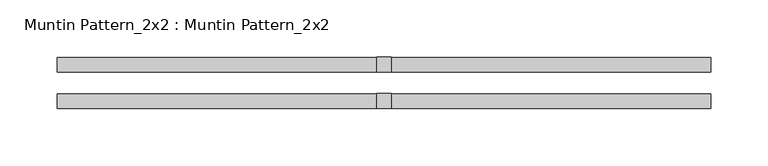
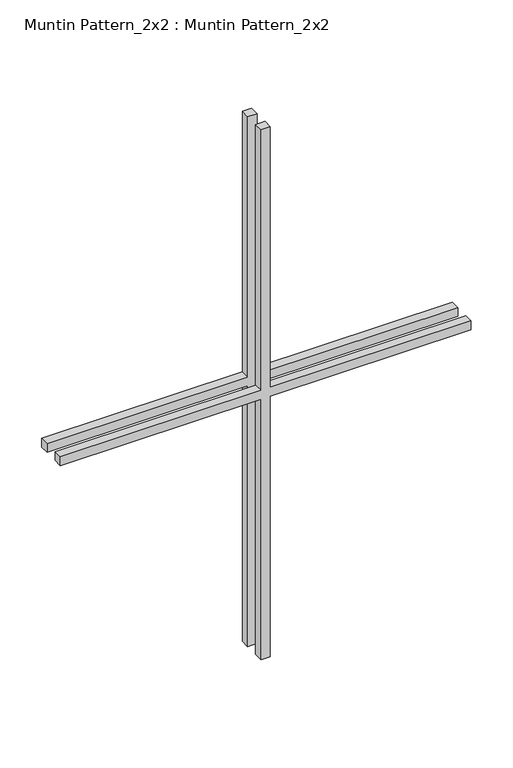
"""IFC4 building model written with IfcOpenShell, lengths in millimetres: proxy geometry, Muntin Pattern_2x2 : Muntin Pattern_2x2."""

from ifc_helpers import new_model, si_unit, frame, origin, place, context, project, spatial, polyline, outline, extrude, source, transform, mapped, element, save


def muntin_pattern_2x2_muntin_pattern_2x2_fbb866f2(model_context):
    return source(origin(), model_context, "Body", "SweptSolid", [
        extrude(outline(polyline([(393.7, -6.35), (393.7, -284.1625), (381.0, -284.1625), (381.0, -6.35), (0.0, -6.35), (0.0, 6.35), (381.0, 6.35), (381.0, 284.1625), (393.7, 284.1625), (393.7, 6.35), (774.7, 6.35), (774.7, -6.35), (393.7, -6.35)])), frame((0.0, -22.225, 0.0), z_axis=(0.0, 1.0, 0.0), x_axis=(0.0, 0.0, 1.0)), (0.0, 0.0, 1.0), 12.7),
        extrude(outline(polyline([(393.7, -6.35), (393.7, -284.1625), (381.0, -284.1625), (381.0, -6.35), (0.0, -6.35), (0.0, 6.35), (381.0, 6.35), (381.0, 284.1625), (393.7, 284.1625), (393.7, 6.35), (774.7, 6.35), (774.7, -6.35), (393.7, -6.35)])), frame((0.0, 9.525, 0.0), z_axis=(0.0, 1.0, 0.0), x_axis=(0.0, 0.0, 1.0)), (0.0, 0.0, 1.0), 12.7),
    ])


if __name__ == "__main__":
    model = new_model("IFC4")
    model_context = context("Model", 3, world=origin())
    ifc_project = project(units=[si_unit("LENGTHUNIT", "METRE", prefix="MILLI")], contexts=[model_context])
    site = spatial("IfcSite", under=ifc_project)
    building = spatial("IfcBuilding", under=site)
    placement = place(None, origin())
    muntin_pattern_2x2_muntin_pattern_2x2_shape = muntin_pattern_2x2_muntin_pattern_2x2_fbb866f2(model_context)
    element("IfcBuildingElementProxy", 1, Name="Muntin Pattern_2x2 : Muntin Pattern_2x2", ObjectType="Muntin Pattern_2x2 : Muntin Pattern_2x2", at=placement, inside=building, context=model_context, shape_type="MappedRepresentation", body=[
        mapped(muntin_pattern_2x2_muntin_pattern_2x2_shape, transform((0.0, 0.0, 0.0), x_axis=(1.0, 0.0, 0.0), y_axis=(0.0, 1.0, 0.0), z_axis=(0.0, 0.0, 1.0))),
    ])
    save(model, "model.ifc")

# Revit data of these elements
# Type "Muntin Pattern_2x2 : Muntin Pattern_2x2"
#   Width [instance default] = 4' - 0"
#   Thickness = 0' - 0 1/2"
#   Height [instance default] = 4' - 0"
#   Distance = 0' - 0 3/4"
#   Interior Material [instance default] = none
#   Exterior Material [instance default] = none
#   Default Elevation = 0
# Element 1 (IfcBuildingElementProxy, "Muntin Pattern_2x2 : Muntin Pattern_2x2")
#   Width = 1' - 10 3/8"
#   Height = 2' - 6 1/2"
#   Interior Material = Wood - Stained
#   Exterior Material = Clad - White
#   Materials on its faces: "Clad - White", "Wood - Stained"
# Materials
#   "Clad - White": class "Wood", colour RGB 242 242 238, transparency 0, Cost = 0
#   "Wood - Stained": class "Wood", colour RGB 224 178 126, transparency 0, Cost = 0
